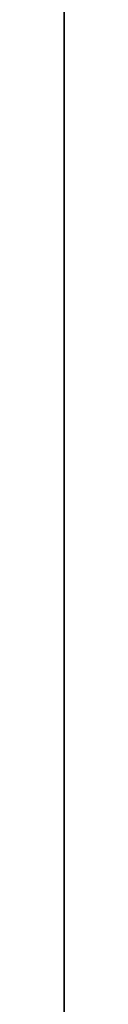
# Model space of a CAD drawing. Units: inches. Extents: x 2083 to 3317, y 1141 to 2115.
# Tile 74 of 256: x 2235.96 to 2235.96, y 1481.434 to 1485.751. Entities that reach past the tile are written whole.
import ezdxf

# ---------------------------------------------------------------- set-up
doc = ezdxf.new("R2010")
doc.units = ezdxf.units.IN
doc.layers.add('A-ANNO-DIMS', color=2, linetype='Continuous', lineweight=18)
doc.layers.add('A-WALL', color=7, linetype='Continuous', lineweight=35)
doc.layers.add('A-WALL-PATT', color=251, linetype='Continuous', lineweight=13, true_color=0x636466)
doc.styles.get("Standard").update_dxf_attribs({"font": 'arial.ttf'})
doc.dimstyles.new('ISO-25', dxfattribs={"dimtxt": 12, "dimasz": 12, "dimexe": 1.25, "dimexo": 0.625, "dimtad": 1, "dimlunit": 3, "dimtxsty": 'Standard', "dimcen": 2.5, "dimadec": 0, "dimazin": 0, "dimtfac": 1, "dimtmove": 0, "dimatfit": 3, "dimfxl": 1, "dimarcsym": 0})

# ---------------------------------------------------------------- blocks, each defined once
blk = doc.blocks.new('*D30')
at = {"layer": 'A-ANNO-DIMS', "color": 0, "lineweight": -2, "transparency": 16777216}
for p, q in [((2240.0179, 1445.2738), (2240.0179, 1448.0455)), ((2254.3293, 1445.2738), (2254.3293, 1448.0455)), ((2228.0179, 1446.7955), (2216.0179, 1446.7955)), ((2240.0179, 1446.7955), (2254.3293, 1446.7955)), ((2266.3293, 1446.7955), (2413.7649, 1446.7955))]:
    blk.add_line(p, q, dxfattribs=at)
at = {"layer": 'A-ANNO-DIMS', "color": 0, "transparency": 16777216}
for points in [[(2228.0179, 1448.7955), (2228.0179, 1444.7955), (2240.0179, 1446.7955)], [(2266.3293, 1448.7955), (2266.3293, 1444.7955), (2254.3293, 1446.7955)]]:
    blk.add_solid(points, dxfattribs=at)
at = {"layer": 'Defpoints', "color": 0, "transparency": 16777216}
for p in [(2254.3293, 1446.7955), (2240.0179, 1444.6488), (2254.3293, 1444.6488)]:
    blk.add_point(p, dxfattribs=at)
at = {"layer": 'A-ANNO-DIMS', "color": 0, "transparency": 16777216, "insert": (2346.0471, 1453.6252), "char_height": 12, "attachment_point": 5}
blk.add_mtext('WC 1\'-2 1/2" TYP.', dxfattribs=at)
blk = doc.blocks.new('*D31')
at = {"layer": 'A-ANNO-DIMS', "color": 0, "lineweight": -2, "transparency": 16777216}
for p, q in [((2237.8711, 1456.6488), (2237.8711, 1541.9152)), ((2239.3929, 1444.6488), (2236.6211, 1444.6488)), ((2237.8711, 1431.5475), (2237.8711, 1444.6488)), ((2239.3929, 1431.5475), (2236.6211, 1431.5475)), ((2237.8711, 1419.5475), (2237.8711, 1407.5475))]:
    blk.add_line(p, q, dxfattribs=at)
at = {"layer": 'A-ANNO-DIMS', "color": 0, "transparency": 16777216}
for points in [[(2235.8711, 1456.6488), (2239.8711, 1456.6488), (2237.8711, 1444.6488)], [(2235.8711, 1419.5475), (2239.8711, 1419.5475), (2237.8711, 1431.5475)]]:
    blk.add_solid(points, dxfattribs=at)
at = {"layer": 'Defpoints', "color": 0, "transparency": 16777216}
for p in [(2237.8711, 1444.6488), (2240.0179, 1444.6488), (2240.0179, 1431.5475)]:
    blk.add_point(p, dxfattribs=at)
at = {"layer": 'A-ANNO-DIMS', "color": 0, "transparency": 16777216, "insert": (2231.2175, 1505.282), "char_height": 12, "attachment_point": 5, "rotation": 90}
blk.add_mtext('1\'-1" TYP.', dxfattribs=at)
blk = doc.blocks.new('*D45')
at = {"layer": 'A-ANNO-DIMS', "color": 0, "lineweight": -2, "transparency": 16777216}
for p, q in [((2235.9598, 1478.3864), (2235.9598, 1531.3614)), ((2418.9598, 1478.3864), (2418.9598, 1531.3614)), ((2247.9598, 1530.1114), (2406.9598, 1530.1114))]:
    blk.add_line(p, q, dxfattribs=at)
at = {"layer": 'A-ANNO-DIMS', "color": 0, "transparency": 16777216}
for points in [[(2247.9598, 1532.1114), (2247.9598, 1528.1114), (2235.9598, 1530.1114)], [(2406.9598, 1532.1114), (2406.9598, 1528.1114), (2418.9598, 1530.1114)]]:
    blk.add_solid(points, dxfattribs=at)
at = {"layer": 'Defpoints', "color": 0, "transparency": 16777216}
for p in [(2418.9598, 1530.1114), (2235.9598, 1477.7614), (2418.9598, 1477.7614)]:
    blk.add_point(p, dxfattribs=at)
at = {"layer": 'A-ANNO-DIMS', "color": 0, "transparency": 16777216, "insert": (2327.4598, 1536.8673), "char_height": 12, "attachment_point": 5}
blk.add_mtext('15\'-3"', dxfattribs=at)
blk = doc.blocks.new('*D62')
at = {"layer": 'A-ANNO-DIMS', "color": 0, "lineweight": -2, "transparency": 16777216}
for p, q in [((2235.9598, 1469.3864), (2235.9598, 1522.3614)), ((2379.9598, 1469.3864), (2379.9598, 1522.3614)), ((2247.9598, 1521.1114), (2367.9598, 1521.1114))]:
    blk.add_line(p, q, dxfattribs=at)
at = {"layer": 'A-ANNO-DIMS', "color": 0, "transparency": 16777216}
for points in [[(2247.9598, 1523.1114), (2247.9598, 1519.1114), (2235.9598, 1521.1114)], [(2367.9598, 1523.1114), (2367.9598, 1519.1114), (2379.9598, 1521.1114)]]:
    blk.add_solid(points, dxfattribs=at)
at = {"layer": 'Defpoints', "color": 0, "transparency": 16777216}
for p in [(2379.9598, 1521.1114), (2235.9598, 1468.7614), (2379.9598, 1468.7614)]:
    blk.add_point(p, dxfattribs=at)
at = {"layer": 'A-ANNO-DIMS', "color": 0, "transparency": 16777216, "insert": (2307.9598, 1527.8632), "char_height": 12, "attachment_point": 5}
blk.add_mtext('12\'-0"', dxfattribs=at)

msp = doc.modelspace()

# ---------------------------------------------------------------- hatches: boundary and pattern name
at = {"layer": 'A-WALL-PATT'}
h = msp.add_hatch(color=256, dxfattribs=at)
h.dxf.hatch_style = 1
h.paths.add_polyline_path([(3126.9598, 2020.7614), (2748.9598, 2020.7614), (2604.9598, 2020.7614), (2226.9598, 2020.7614), (2226.9598, 1702.7614), (2466.9598, 1702.7614), (2466.9598, 1582.7614), (2418.9598, 1582.7614), (2418.9598, 1477.7614), (2226.9598, 1477.7614), (2226.9598, 1263.2614), (2544.9598, 1263.2614), (2544.9598, 1411.7614), (2604.9598, 1411.7614), (2685.9598, 1411.7614), (2685.9598, 1420.7614), (2604.9598, 1420.7614), (2604.9598, 1573.7614), (2604.9598, 1702.7614), (2604.9598, 2011.7614), (2748.9598, 2011.7614), (2748.9598, 1702.7614), (2862.9598, 1702.7614), (2862.9598, 1621.7614), (2871.9598, 1621.7614), (2871.9598, 1702.7614), (2883.9598, 1702.7614), (2883.9598, 1706.9395, -0.026459), (2883.9598, 1711.7614), (2757.9598, 1711.7614), (2757.9598, 1807.7614), (2787.9598, 1807.7614), (2787.9598, 1812.2614), (2757.9598, 1812.2614), (2757.9598, 2011.7614), (2877.9598, 2011.7614), (2877.9598, 1812.2614), (2847.9598, 1812.2614), (2847.9598, 1807.7614), (2889.8357, 1807.7614), (2889.8357, 1812.2614), (2882.4598, 1812.2614), (2882.4598, 2011.7614), (3117.9598, 2011.7614), (3117.9598, 1812.2614), (2937.8357, 1812.2614), (2937.8357, 1807.7614), (2995.7098, 1807.7614), (2995.7098, 1796.1177), (3000.2098, 1796.1177), (3000.2098, 1807.7614), (3117.9598, 1807.7614), (3117.9598, 1711.7614), (3000.2098, 1711.7614), (3000.2098, 1760.1177), (2998.5727, 1760.1177, -0.020711), (2995.7098, 1760.1177), (2995.7098, 1711.7614), (2931.9598, 1711.7614), (2931.9598, 1702.7614), (3126.9598, 1702.7614)])
h.paths.add_polyline_path([(2471.4598, 2011.7614), (2471.4598, 1810.0114), (2462.7169, 1810.0114), (2462.7169, 1805.5114), (2505.9598, 1805.5114), (2505.9598, 1810.0114), (2475.9598, 1810.0114), (2475.9598, 2011.7614), (2595.9598, 2011.7614), (2595.9598, 1810.0114), (2565.9598, 1810.0114), (2565.9598, 1805.5114), (2595.9598, 1805.5114), (2595.9598, 1711.7614), (2235.9598, 1711.7614), (2235.9598, 1805.5114), (2353.7098, 1805.5114), (2353.7098, 1796.0542), (2358.2098, 1796.0542), (2358.2098, 1805.5114), (2414.7169, 1805.5114), (2414.7169, 1810.0114), (2235.9598, 1810.0114), (2235.9598, 2011.7614)], flags=16)
h.paths.add_polyline_path([(2270.2047, 1994.61), (2270.2047, 1970.61), (2246.2047, 1970.61), (2246.2047, 1994.61)], flags=0)
edge = h.paths.add_edge_path(flags=0)
edge.add_ellipse((2332.0274, 1899.7982), major_axis=(-3.043, 3.043), ratio=0.168252, start_angle=-161.3322, end_angle=-156.3071, ccw=False)
edge.add_ellipse((2333.082, 1898.7435), major_axis=(-1.0546, 1.0546), ratio=0.453532, start_angle=-123.371, end_angle=-94.1591)
edge = h.paths.add_edge_path(flags=0)
edge.add_ellipse((2332.0274, 1968.8763), major_axis=(3.043, 3.043), ratio=0.168252, start_angle=18.6678, end_angle=23.6929)
edge.add_spline(control_points=[(2332.9256, 1970.6911), (2332.2268, 1970.3361), (2330.8937, 1969.6589), (2328.4131, 1970.9321), (2327.2039, 1967.7487), (2324.7096, 1969.9556), (2322.5328, 1967.0124), (2320.0128, 1971.2958), (2317.6803, 1968.1578), (2316.0405, 1967.102), (2315.4269, 1966.8096)], knot_values=[0, 0, 0, 0, 2.267059, 4.324559, 6.685584, 8.878641, 11.121502, 14.300359, 17.755284, 19.732645, 19.732645, 19.732645, 19.732645], degree=3, periodic=0)
edge.add_ellipse((2332.0274, 1968.8763), major_axis=(3.043, 3.043), ratio=0.168252, start_angle=18.6678, end_angle=23.6929, ccw=False)
edge.add_ellipse((2333.082, 1969.9309), major_axis=(1.0546, 1.0546), ratio=0.453532, start_angle=56.629, end_angle=85.8409, ccw=False)
edge = h.paths.add_edge_path(flags=0)
edge.add_spline(control_points=[(2296.4283, 1967.9879), (2293.6278, 1965.3363), (2287.7036, 1959.7271), (2299.7439, 1949.9957), (2294.5326, 1935.6685), (2290.5732, 1920.6035), (2293.3941, 1909.9737), (2296.1854, 1904.9665)], knot_values=[0.099185, 0.099185, 0.099185, 0.099185, 0.345301, 0.619822, 0.982653, 1.386093, 1.810555, 1.810555, 1.810555, 1.810555], degree=3, periodic=0)
edge.add_spline(control_points=[(2296.1854, 1904.9665), (2297.3836, 1902.6193), (2298.001, 1901.9493), (2298.553, 1901.4682)], knot_values=[0.006246, 0.006246, 0.006246, 0.006246, 0.055476, 0.055476, 0.055476, 0.055476], degree=3, periodic=0)
edge.add_spline(control_points=[(2298.553, 1901.4682), (2297.2586, 1900.9232), (2295.2253, 1900.2321), (2293.0602, 1900.6142), (2292.1014, 1900.7884), (2292.0896, 1900.7906)], knot_values=[0.312835, 0.312835, 0.312835, 0.312835, 0.40178, 0.474987, 0.475903, 0.475903, 0.475903, 0.475903], degree=3, periodic=0)
edge.add_arc((2292.7936, 1904.6641), 3.937, 215.4209, 259.6982, ccw=False)
edge.add_spline(control_points=[(2289.5853, 1902.3823), (2289.4767, 1902.5351), (2289.3685, 1902.688), (2289.2609, 1902.8412)], knot_values=[0.102872, 0.102872, 0.102872, 0.102872, 0.116896, 0.116896, 0.116896, 0.116896], degree=3, periodic=0)
edge.add_spline(control_points=[(2289.2609, 1902.8412), (2288.6866, 1902.5502), (2287.64, 1902.0199), (2285.8813, 1901.874), (2283.853, 1901.5044), (2281.72, 1899.7105), (2278.467, 1899.4929), (2276.1571, 1901.8832), (2272.259, 1899.8041), (2267.7776, 1901.8432), (2262.2439, 1900.184), (2257.4149, 1901.7821), (2254.3184, 1900.7261), (2253.1783, 1900.3373)], knot_values=[0, 0, 0, 0, 1.907977, 3.477176, 5.261074, 7.972851, 11.680248, 13.717921, 16.939592, 22.789562, 27.502503, 33.595215, 37.145618, 37.145618, 37.145618, 37.145618], degree=3, periodic=0)
edge.add_line((2253.1783, 1900.3373), (2250.2442, 1902.8412))
edge.add_line((2250.2442, 1902.8412), (2250.2442, 1965.8333))
edge.add_line((2250.2442, 1965.8333), (2253.1783, 1968.3371))
edge.add_spline(control_points=[(2253.1783, 1968.3371), (2254.3184, 1967.9483), (2257.4149, 1966.8924), (2262.2439, 1968.4904), (2267.7776, 1966.8313), (2271.5267, 1968.5372), (2273.8759, 1967.8283), (2274.2067, 1967.7276)], knot_values=[0, 0, 0, 0, 0.09018, 0.244935, 0.364644, 0.513233, 0.537855, 0.537855, 0.537855, 0.537855], degree=3, periodic=0)
edge.add_arc((2274.3529, 1963.7933), 3.937, 72.0511, 92.1279, ccw=False)
edge.add_arc((2281.2969, 1985.23), 18.5963, 252.05113, 288.56572)
edge.add_arc((2292.3167, 1956.0289), 12.6461, 71.02679, 113.77822, ccw=False)
edge = h.paths.add_edge_path(flags=0)
edge.add_spline(control_points=[(2274.8994, 1951.8562), (2275.0662, 1951.6166), (2275.2327, 1951.3766), (2275.398, 1951.1359)], knot_values=[1.409916, 1.409916, 1.409916, 1.409916, 1.43159, 1.43159, 1.43159, 1.43159], degree=3, periodic=0)
edge.add_spline(control_points=[(2275.398, 1951.1359), (2275.7921, 1950.5619), (2276.1792, 1949.9838), (2276.5455, 1949.3971)], knot_values=[1.358238, 1.358238, 1.358238, 1.358238, 1.409916, 1.409916, 1.409916, 1.409916], degree=3, periodic=0)
edge.add_line((2276.5455, 1949.3971), (2277.4373, 1947.8622))
edge.add_spline(control_points=[(2277.4373, 1947.8622), (2276.3038, 1945.6731), (2274.6397, 1942.4269), (2274.6316, 1938.0939), (2272.7991, 1930.8515), (2274.3564, 1943.897), (2275.9477, 1947.9234), (2276.5455, 1949.3971)], knot_values=[0.005632, 0.005632, 0.005632, 0.005632, 0.186014, 0.266002, 0.357087, 0.59639, 0.739732, 0.739732, 0.739732, 0.739732], degree=3, periodic=0)
edge.add_spline(control_points=[(2276.5455, 1949.3971), (2276.1792, 1949.9838), (2275.7921, 1950.5619), (2275.398, 1951.1359)], knot_values=[1.358238, 1.358238, 1.358238, 1.358238, 1.409916, 1.409916, 1.409916, 1.409916], degree=3, periodic=0)
edge.add_spline(control_points=[(2275.398, 1951.1359), (2274.9425, 1950.0805), (2274.2078, 1948.0253), (2273.9346, 1944.8515), (2272.4685, 1937.6275), (2273.4662, 1945.6965), (2274.7006, 1951.0595), (2274.8994, 1951.8562)], knot_values=[0.104364, 0.104364, 0.104364, 0.104364, 0.189636, 0.269624, 0.36071, 0.600013, 0.644622, 0.644622, 0.644622, 0.644622], degree=3, periodic=0)
h.paths.add_polyline_path([(2269.1675, 1963.1276, -0.357527), (2268.1706, 1960.9764, -0.092561), (2268.1706, 1939.4363, -0.357527), (2269.1675, 1937.2851, -0.357527), (2267.0163, 1938.282, -0.164785), (2254.6856, 1938.282, -0.357527), (2252.5344, 1937.2851, -0.357527), (2253.5313, 1939.4363, -0.092561), (2253.5313, 1960.9764, -0.357527), (2252.5344, 1963.1276, -0.357527), (2254.6856, 1962.1307, -0.164785), (2267.0163, 1962.1307, -0.357527)], flags=0)
h.paths.add_polyline_path([(2248.8741, 1967.8018), (2248.8741, 1957.0277), (2249.4578, 1957.0277), (2249.4578, 1911.6468), (2248.8741, 1911.6468), (2248.8741, 1900.8727), (2246.5119, 1900.8727, 0.197327), (2244.1497, 1902.4569), (2244.1497, 1966.2176, 0.197327), (2246.5119, 1967.8018)], flags=0)
h.paths.add_polyline_path([(2269.1675, 1931.3893, -0.357527), (2268.1706, 1929.2381, -0.092561), (2268.1706, 1907.6981, -0.357527), (2269.1675, 1905.5469, -0.357527), (2267.0163, 1906.5438, -0.164785), (2254.6856, 1906.5438, -0.357527), (2252.5344, 1905.5469, -0.357527), (2253.5313, 1907.6981, -0.092561), (2253.5313, 1929.2381, -0.357527), (2252.5344, 1931.3893, -0.357527), (2254.6856, 1930.3925, -0.164785), (2267.0163, 1930.3925, -0.357527)], flags=0)
edge = h.paths.add_edge_path(flags=0)
edge.add_spline(control_points=[(2276.1969, 1906.7237), (2276.1681, 1909.0289), (2276.114, 1913.3719), (2270.5984, 1924.925), (2273.9052, 1919.0128), (2275.9217, 1916.2621), (2275.4746, 1912.4021), (2277.2579, 1910.3806), (2276.696, 1908.225), (2276.6462, 1906.813), (2276.6178, 1906.0084)], knot_values=[0, 0, 0, 0, 8.61026, 16.221274, 18.843057, 23.804898, 27.440828, 29.356102, 31.203478, 33.650687, 33.650687, 33.650687, 33.650687], degree=3, periodic=0)
edge.add_spline(control_points=[(2276.6178, 1906.0084), (2276.6233, 1905.6241), (2276.4977, 1904.6287), (2275.4418, 1903.8547), (2274.9373, 1903.0804), (2274.8591, 1902.8412)], knot_values=[0.156488, 0.156488, 0.156488, 0.156488, 0.184398, 0.231376, 0.250598, 0.250598, 0.250598, 0.250598], degree=3, periodic=0)
edge.add_line((2274.8591, 1902.8412), (2276.506, 1902.8412))
edge.add_spline(control_points=[(2276.506, 1902.8412), (2276.7883, 1903.0849), (2277.6651, 1904.1252), (2278.2495, 1904.3407), (2277.6539, 1908.5274), (2278.1557, 1906.2278), (2278.1005, 1905.2859), (2278.8467, 1904.069), (2277.8568, 1903.4149), (2277.8742, 1902.991), (2277.9036, 1902.8412)], knot_values=[0.059574, 0.059574, 0.059574, 0.059574, 0.080753, 0.103741, 0.16972, 0.176036, 0.207137, 0.240474, 0.262341, 0.27366, 0.27366, 0.27366, 0.27366], degree=3, periodic=0)
edge.add_line((2277.9036, 1902.8412), (2280.0298, 1902.8412))
edge.add_spline(control_points=[(2280.0298, 1902.8412), (2279.8882, 1903.0884), (2279.4993, 1903.9816), (2280.1523, 1905.9393), (2278.1036, 1909.6578), (2279.7624, 1907.1853), (2280.3279, 1904.8749), (2280.4851, 1903.4896), (2281.4633, 1903.2494), (2281.7583, 1902.9365), (2281.834, 1902.8412)], knot_values=[0.013856, 0.013856, 0.013856, 0.013856, 0.034874, 0.088867, 0.107879, 0.126738, 0.158714, 0.193757, 0.217487, 0.226722, 0.226722, 0.226722, 0.226722], degree=3, periodic=0)
edge.add_spline(control_points=[(2281.834, 1902.8412), (2281.7875, 1902.8267), (2281.647, 1902.783), (2281.3955, 1902.8595), (2281.0881, 1902.9852), (2280.7207, 1903.0609), (2280.3335, 1903.0257), (2280.1248, 1902.8989), (2280.0298, 1902.8412)], knot_values=[0, 0, 0, 0, 0.14413, 0.435517, 0.749276, 1.153046, 1.548371, 1.878348, 1.878348, 1.878348, 1.878348], degree=3, periodic=0)
edge.add_line((2280.0298, 1902.8412), (2277.9036, 1902.8412))
edge.add_spline(control_points=[(2277.9036, 1902.8412), (2277.8929, 1902.7959), (2277.8654, 1902.6796), (2277.6075, 1902.6875), (2277.2741, 1902.8007), (2276.8379, 1902.6198), (2276.5838, 1902.7893), (2276.506, 1902.8412)], knot_values=[0, 0, 0, 0, 0.127189, 0.326199, 0.628009, 1.24357, 1.515331, 1.515331, 1.515331, 1.515331], degree=3, periodic=0)
edge.add_line((2276.506, 1902.8412), (2274.8591, 1902.8412))
edge.add_spline(control_points=[(2274.8591, 1902.8412), (2274.8144, 1902.8986), (2274.7251, 1903.0134), (2274.4935, 1903.119), (2274.2443, 1902.9605), (2273.9371, 1903.1849), (2273.614, 1902.9831), (2273.4083, 1902.883), (2273.3223, 1902.8412)], knot_values=[0, 0, 0, 0, 0.21843, 0.436957, 0.687977, 0.990379, 1.398396, 1.69185, 1.69185, 1.69185, 1.69185], degree=3, periodic=0)
edge.add_spline(control_points=[(2273.3223, 1902.8412), (2273.6167, 1903.4457), (2274.274, 1904.5383), (2276.0272, 1904.5737), (2276.207, 1906.5836), (2276.1969, 1906.7237)], knot_values=[0.012227, 0.012227, 0.012227, 0.012227, 0.059472, 0.106218, 0.134458, 0.134458, 0.134458, 0.134458], degree=3, periodic=0)
h.paths.add_polyline_path([(2270.7761, 1897.7898), (2270.7761, 1873.7898), (2246.7761, 1873.7898), (2246.7761, 1897.7898)], flags=0)
h.paths.add_polyline_path([(2353.7098, 1760.0051), (2353.7098, 1760.0542), (2358.2098, 1760.0542, -0.033729)], flags=0)
h.paths.add_polyline_path([(2321.8191, 1737.5292), (2341.9953, 1737.5292, -0.414214), (2343.2033, 1736.3212), (2343.2033, 1721.0206, -0.414214), (2341.9953, 1719.8127), (2321.8191, 1719.8127, -0.414214), (2320.6112, 1721.0206), (2320.6112, 1736.3212, -0.414214)], flags=0)
h.paths.add_polyline_path([(2324.235, 1736.3212), (2339.5794, 1736.3212, -0.414214), (2341.9953, 1733.9053), (2341.9953, 1725.4497, -0.414214), (2339.5794, 1723.0338), (2333.6806, 1723.0338), (2333.8453, 1722.0455, -0.870646), (2335.4254, 1721.8259, -0.767327), (2333.9227, 1721.4232), (2331.291, 1721.4232, -0.767327), (2329.7883, 1721.8259, -0.870646), (2331.3684, 1722.0455), (2331.5331, 1723.0338), (2324.235, 1723.0338, -0.414214), (2321.8191, 1725.4497), (2321.8191, 1733.9053, -0.414214)], flags=0)
h.paths.add_polyline_path([(2570.4838, 1928.6154), (2589.6838, 1928.6154), (2590.1688, 1928.6154), (2590.1688, 1904.9934), (2570.4838, 1904.9934)], flags=0)
h.paths.add_polyline_path([(2574.4473, 1927.2638, -1), (2572.8288, 1927.2638, -1)], flags=0)
h.paths.add_polyline_path([(2573.0899, 1926.9409), (2573.925, 1927.776), (2574.1477, 1927.5533), (2573.3126, 1926.7182)], flags=0)
h.paths.add_polyline_path([(2578.7791, 1919.7296, -1), (2571.5917, 1919.7296, -1)], flags=0)
h.paths.add_polyline_path([(2578.3854, 1919.7296, -1), (2571.9854, 1919.7296, -1)], flags=0)
h.paths.add_polyline_path([(2331.5958, 1729.4762, -1), (2333.618, 1729.4762, -1)], flags=0)
h.paths.add_polyline_path([(2578.0342, 1927.2638, -1), (2576.4157, 1927.2638, -1)], flags=0)
h.paths.add_polyline_path([(2576.6889, 1927.5311), (2576.9116, 1927.7538), (2577.7467, 1926.9186), (2577.524, 1926.6959)], flags=0)
h.paths.add_polyline_path([(2578.1391, 1909.8595, -1), (2572.2317, 1909.8595, -1)], flags=0)
h.paths.add_polyline_path([(2577.7454, 1909.8595, -1), (2572.6254, 1909.8595, -1)], flags=0)
h.paths.add_polyline_path([(2583.7977, 1927.2638, -1), (2582.1792, 1927.2638, -1)], flags=0)
h.paths.add_polyline_path([(2582.7186, 1927.7538), (2583.5538, 1926.9186), (2583.3311, 1926.6959), (2582.4959, 1927.5311)], flags=0)
h.paths.add_polyline_path([(2582.4959, 1927.5311), (2582.7186, 1927.7538), (2583.5538, 1926.9186), (2583.3311, 1926.6959)], flags=0)
h.paths.add_polyline_path([(2587.7391, 1920.5296, -1), (2581.8317, 1920.5296, -1)], flags=0)
h.paths.add_polyline_path([(2587.3454, 1920.5296, -1), (2582.2254, 1920.5296, -1)], flags=0)
h.paths.add_polyline_path([(2587.3846, 1927.2638, -1), (2585.7661, 1927.2638, -1)], flags=0)
h.paths.add_polyline_path([(2586.082, 1926.9802), (2586.9172, 1927.8154), (2587.1399, 1927.5927), (2586.3047, 1926.7575)], flags=0)
h.paths.add_polyline_path([(2588.3791, 1910.6595, -1), (2581.1917, 1910.6595, -1)], flags=0)
h.paths.add_polyline_path([(2587.9854, 1910.6595, -1), (2581.5854, 1910.6595, -1)], flags=0)
h.paths.add_polyline_path([(2417.1677, 1729.4779), (2437.3439, 1729.4779, -0.414214), (2438.5519, 1728.2699), (2438.5519, 1712.9693, -0.414214), (2437.3439, 1711.7614), (2417.1677, 1711.7614, -0.414214), (2415.9598, 1712.9693), (2415.9598, 1728.2699, -0.414214)], flags=0)
h.paths.add_polyline_path([(2419.5836, 1728.2699), (2434.928, 1728.2699, -0.414214), (2437.3439, 1725.8541), (2437.3439, 1717.3984, -0.414214), (2434.928, 1714.9825), (2429.0292, 1714.9825), (2429.1939, 1713.9942, -0.870646), (2430.774, 1713.7746, -0.767327), (2429.2713, 1713.372), (2426.6396, 1713.372, -0.767327), (2425.1369, 1713.7746, -0.870646), (2426.717, 1713.9942), (2426.8817, 1714.9825), (2419.5836, 1714.9825, -0.414214), (2417.1677, 1717.3984), (2417.1677, 1725.8541, -0.414214)], flags=0)
h.paths.add_polyline_path([(2419.5836, 1728.2699), (2434.928, 1728.2699, -0.414214), (2437.3439, 1725.8541), (2437.3439, 1717.3984, -0.414214), (2434.928, 1714.9825), (2429.0292, 1714.9825), (2428.3581, 1719.009), (2427.5528, 1719.009), (2426.8817, 1714.9825), (2419.5836, 1714.9825, -0.414214), (2417.1677, 1717.3984), (2417.1677, 1725.8541, -0.414214)], flags=0)
h.paths.add_polyline_path([(2426.9444, 1721.4249, -1), (2428.9666, 1721.4249, -1)], flags=0)
h.paths.add_polyline_path([(2475.9598, 1702.7614), (2595.9598, 1702.7614), (2595.9598, 1582.7614), (2475.9598, 1582.7614)], flags=16)
h.paths.add_polyline_path([(2427.9598, 1573.7614), (2595.9598, 1573.7614), (2595.9598, 1468.7614), (2595.9598, 1420.7614), (2384.4598, 1420.7614), (2384.4598, 1468.7614), (2427.9598, 1468.7614)], flags=16)
h.paths.add_polyline_path([(2379.9598, 1468.7614), (2379.9598, 1420.7614), (2235.9598, 1420.7614), (2235.9598, 1468.7614)], flags=16)
h.paths.add_polyline_path([(2317.816, 1466.6958), (2337.9922, 1466.6958, -0.414214), (2339.2002, 1465.4878), (2339.2002, 1450.1872, -0.414214), (2337.9922, 1448.9792), (2317.816, 1448.9792, -0.414214), (2316.6081, 1450.1872), (2316.6081, 1465.4878, -0.414214)], flags=0)
h.paths.add_polyline_path([(2320.2319, 1465.4878), (2335.5763, 1465.4878, -0.414214), (2337.9922, 1463.0719), (2337.9922, 1454.6163, -0.414214), (2335.5763, 1452.2004), (2329.6775, 1452.2004), (2329.8422, 1451.212, -0.870646), (2331.4223, 1450.9925, -0.767327), (2329.9196, 1450.5898), (2327.2879, 1450.5898, -0.767327), (2325.7852, 1450.9925, -0.870646), (2327.3653, 1451.212), (2327.53, 1452.2004), (2320.2319, 1452.2004, -0.414214), (2317.816, 1454.6163), (2317.816, 1463.0719, -0.414214)], flags=0)
h.paths.add_polyline_path([(2320.2319, 1465.4878), (2335.5763, 1465.4878, -0.414214), (2337.9922, 1463.0719), (2337.9922, 1454.6163, -0.414214), (2335.5763, 1452.2004), (2329.6775, 1452.2004), (2329.0064, 1456.2269), (2328.2011, 1456.2269), (2327.53, 1452.2004), (2320.2319, 1452.2004, -0.414214), (2317.816, 1454.6163), (2317.816, 1463.0719, -0.414214)], flags=0)
h.paths.add_polyline_path([(2327.5926, 1458.6428, -1), (2329.6148, 1458.6428, -1)], flags=0)
h.paths.add_polyline_path([(2244.4117, 1433.3405), (2241.9209, 1433.3405, -0.414214), (2240.0179, 1435.2435), (2240.0179, 1440.9528, -0.414211), (2241.9209, 1442.8559), (2244.4117, 1442.8559, -1.976472)], flags=0)
h.paths.add_polyline_path([(2245.3569, 1434.3975, -0.414214), (2245.3569, 1441.7988, -2.144098)], flags=0)
h.paths.add_polyline_path([(2535.9598, 1416.2614), (2535.9598, 1272.2614), (2235.9598, 1272.2614), (2235.9598, 1416.2614)], flags=16)
h.paths.add_polyline_path([(2260.1196, 1384.2928), (2260.1196, 1362.0386), (2237.8654, 1362.0386), (2237.8654, 1384.2928)], flags=0)
edge = h.paths.add_edge_path(flags=0)
edge.add_line((2318.2518, 1362.0933), (2318.1458, 1362.001))
edge.add_ellipse((2317.4451, 1360.431), major_axis=(2.8216, 2.8216), ratio=0.168252, start_angle=18.6678, end_angle=20.9481, ccw=False)
edge.add_ellipse((2318.423, 1361.409), major_axis=(0.9779, 0.9779), ratio=0.453532, start_angle=56.629, end_angle=70.2262, ccw=False)
edge = h.paths.add_edge_path(flags=0)
edge.add_line((2319.1074, 1295.5711), (2319.015, 1295.6771))
edge.add_ellipse((2317.4451, 1296.3778), major_axis=(-2.8216, 2.8216), ratio=0.168252, start_angle=-161.3322, end_angle=-159.0519, ccw=False)
edge.add_ellipse((2318.423, 1295.3999), major_axis=(-0.9779, 0.9779), ratio=0.453532, start_angle=-123.371, end_angle=-109.7738)
edge = h.paths.add_edge_path(flags=0)
edge.add_spline(control_points=[(2284.2103, 1301.1702), (2284.5807, 1300.4447), (2284.8912, 1299.892), (2285.1596, 1299.461)], knot_values=[0.039066, 0.039066, 0.039066, 0.039066, 0.055476, 0.055476, 0.055476, 0.055476], degree=3, periodic=0)
edge.add_line((2285.1596, 1299.461), (2284.2103, 1301.1702))
edge = h.paths.add_edge_path(flags=0)
edge.add_line((2280.4125, 1297.298), (2283.37, 1297.0361))
edge.add_line((2283.37, 1297.0361), (2286.4057, 1297.9263))
edge.add_spline(control_points=[(2286.4057, 1297.9263), (2285.3055, 1297.4631), (2284.3448, 1297.1292), (2283.37, 1297.0361)], knot_values=[0.394369, 0.394369, 0.394369, 0.394369, 0.475903, 0.475903, 0.475903, 0.475903], degree=3, periodic=0)
edge.add_spline(control_points=[(2283.37, 1297.0361), (2283.2814, 1297.0277), (2282.3163, 1296.9573), (2281.3125, 1297.1345), (2280.4234, 1297.296), (2280.4125, 1297.298)], knot_values=[0.312835, 0.312835, 0.312835, 0.312835, 0.320246, 0.393453, 0.394369, 0.394369, 0.394369, 0.394369], degree=3, periodic=0)
edge = h.paths.add_edge_path(flags=0)
edge.add_line((2284.4356, 1359.6073), (2280.4463, 1355.328))
edge.add_line((2280.4463, 1355.328), (2279.58, 1351.0178))
edge.add_line((2279.58, 1351.0178), (2282.413, 1346.5804))
edge.add_spline(control_points=[(2282.413, 1346.5804), (2283.1533, 1345.5892), (2284.2529, 1344.0289), (2284.801, 1342.3872), (2284.9352, 1341.8055)], knot_values=[1.240098, 1.240098, 1.240098, 1.240098, 1.332892, 1.382712, 1.382712, 1.382712, 1.382712], degree=3, periodic=0)
edge.add_spline(control_points=[(2284.9352, 1341.8055), (2285.3191, 1340.1406), (2285.233, 1338.4092), (2284.9099, 1336.6541)], knot_values=[1.097484, 1.097484, 1.097484, 1.097484, 1.240098, 1.240098, 1.240098, 1.240098], degree=3, periodic=0)
edge.add_spline(control_points=[(2284.9099, 1336.6541), (2284.5868, 1334.899), (2284.0267, 1333.1203), (2283.4626, 1331.3606)], knot_values=[0.95487, 0.95487, 0.95487, 0.95487, 1.097484, 1.097484, 1.097484, 1.097484], degree=3, periodic=0)
edge.add_line((2283.4626, 1331.3606), (2281.8904, 1326.1534))
edge.add_line((2281.8904, 1326.1534), (2280.7563, 1321.0561))
edge.add_line((2280.7563, 1321.0561), (2280.2992, 1316.002))
edge.add_line((2280.2992, 1316.002), (2280.7159, 1310.9501))
edge.add_line((2280.7159, 1310.9501), (2282.0281, 1305.9721))
edge.add_line((2282.0281, 1305.9721), (2284.2103, 1301.1702))
edge.add_spline(control_points=[(2284.2103, 1301.1702), (2283.3407, 1302.7302), (2282.6119, 1304.3365), (2282.0281, 1305.9721)], knot_values=[0.099185, 0.099185, 0.099185, 0.099185, 0.241799, 0.241799, 0.241799, 0.241799], degree=3, periodic=0)
edge.add_spline(control_points=[(2282.0281, 1305.9721), (2281.4443, 1307.6078), (2281.0055, 1309.2728), (2280.7159, 1310.9501)], knot_values=[0.241799, 0.241799, 0.241799, 0.241799, 0.384413, 0.384413, 0.384413, 0.384413], degree=3, periodic=0)
edge.add_spline(control_points=[(2280.7159, 1310.9501), (2280.4332, 1312.5876), (2280.2894, 1314.277), (2280.2989, 1315.962), (2280.2992, 1316.002)], knot_values=[0.384413, 0.384413, 0.384413, 0.384413, 0.523647, 0.527028, 0.527028, 0.527028, 0.527028], degree=3, periodic=0)
edge.add_spline(control_points=[(2280.2992, 1316.002), (2280.3123, 1317.687), (2280.4779, 1319.3679), (2280.7563, 1321.0561)], knot_values=[0.527028, 0.527028, 0.527028, 0.527028, 0.669642, 0.669642, 0.669642, 0.669642], degree=3, periodic=0)
edge.add_spline(control_points=[(2280.7563, 1321.0561), (2281.0346, 1322.7443), (2281.4259, 1324.4396), (2281.8904, 1326.1534)], knot_values=[0.669642, 0.669642, 0.669642, 0.669642, 0.812256, 0.812256, 0.812256, 0.812256], degree=3, periodic=0)
edge.add_spline(control_points=[(2281.8904, 1326.1534), (2282.2644, 1327.5333), (2282.7879, 1329.2618), (2283.3528, 1331.0178), (2283.4626, 1331.3606)], knot_values=[0.812256, 0.812256, 0.812256, 0.812256, 0.927087, 0.95487, 0.95487, 0.95487, 0.95487], degree=3, periodic=0)
edge.add_line((2283.4626, 1331.3606), (2284.9099, 1336.6541))
edge.add_line((2284.9099, 1336.6541), (2284.9352, 1341.8055))
edge.add_line((2284.9352, 1341.8055), (2282.413, 1346.5804))
edge.add_spline(control_points=[(2282.413, 1346.5804), (2281.2751, 1348.1038), (2280.0784, 1349.5703), (2279.58, 1351.0178)], knot_values=[1.382712, 1.382712, 1.382712, 1.382712, 1.525326, 1.525326, 1.525326, 1.525326], degree=3, periodic=0)
edge.add_spline(control_points=[(2279.58, 1351.0178), (2279.4433, 1351.4147), (2279.1363, 1352.8569), (2279.7352, 1354.2904), (2280.4463, 1355.328)], knot_values=[1.525326, 1.525326, 1.525326, 1.525326, 1.564439, 1.667941, 1.667941, 1.667941, 1.667941], degree=3, periodic=0)
edge.add_spline(control_points=[(2280.4463, 1355.328), (2281.4261, 1356.7578), (2282.9308, 1358.1826), (2284.4356, 1359.6073)], knot_values=[1.667941, 1.667941, 1.667941, 1.667941, 1.810555, 1.810555, 1.810555, 1.810555], degree=3, periodic=0)
edge.add_arc((2280.6231, 1348.5182), 11.7262, 71.02679, 113.77822)
edge.add_arc((2270.4049, 1375.5952), 17.2436, 252.05113, 288.56572, ccw=False)
edge.add_arc((2263.966, 1355.7178), 3.6506, 72.0511, 92.1279)
edge.add_arc((2263.966, 1355.7178), 3.6506, 92.1279, 177.9851)
edge.add_spline(control_points=[(2260.3176, 1355.8462), (2260.2604, 1354.2207), (2260.5513, 1350.1865), (2262.9993, 1346.7663), (2264.4727, 1344.649)], knot_values=[1.43159, 1.43159, 1.43159, 1.43159, 1.564144, 1.770695, 1.770695, 1.770695, 1.770695], degree=3, periodic=0)
edge.add_line((2264.4727, 1344.649), (2264.9356, 1343.9825))
edge.add_spline(control_points=[(2263.801, 1340.2481), (2263.8432, 1340.5141), (2264.0672, 1341.7565), (2264.5127, 1343.0025), (2264.935, 1343.9811)], knot_values=[0.53657, 0.53657, 0.53657, 0.53657, 0.559349, 0.644622, 0.644622, 0.644622, 0.644622], degree=3, periodic=0)
edge.add_spline(control_points=[(2264.935, 1343.9811), (2265.1178, 1343.715), (2265.2989, 1343.4479), (2265.4768, 1343.1794)], knot_values=[1.384077, 1.384077, 1.384077, 1.384077, 1.409916, 1.409916, 1.409916, 1.409916], degree=3, periodic=0)
edge.add_spline(control_points=[(2265.4768, 1343.1794), (2265.6546, 1342.9108), (2265.8293, 1342.6408), (2265.9991, 1342.3688)], knot_values=[1.358238, 1.358238, 1.358238, 1.358238, 1.384077, 1.384077, 1.384077, 1.384077], degree=3, periodic=0)
edge.add_line((2265.9991, 1342.3688), (2266.826, 1340.9455))
edge.add_spline(control_points=[(2266.826, 1340.9455), (2268.8944, 1337.0897), (2271.3982, 1325.843), (2270.5162, 1310.5686), (2275.9194, 1301.8606), (2277.7895, 1299.1994)], knot_values=[0.116896, 0.116896, 0.116896, 0.116896, 0.472987, 1.050969, 1.313793, 1.313793, 1.313793, 1.313793], degree=3, periodic=0)
edge.add_spline(control_points=[(2277.7895, 1299.1994), (2277.8394, 1299.1285), (2277.8894, 1299.0575), (2277.9396, 1298.9866)], knot_values=[0.109884, 0.109884, 0.109884, 0.109884, 0.116896, 0.116896, 0.116896, 0.116896], degree=3, periodic=0)
edge.add_line((2277.9396, 1298.9866), (2277.7888, 1299.1991))
edge.add_spline(control_points=[(2277.7888, 1299.1991), (2277.2566, 1298.9294), (2276.2864, 1298.4379), (2275.0394, 1298.3344), (2274.3833, 1298.2389), (2274.2153, 1298.2093)], knot_values=[33.12187, 33.12187, 33.12187, 33.12187, 35.029056, 36.598255, 37.144827, 37.144827, 37.144827, 37.144827], degree=3, periodic=0)
edge.add_line((2274.2153, 1298.2093), (2273.0731, 1297.893))
edge.add_spline(control_points=[(2273.0731, 1297.893), (2272.3229, 1297.5798), (2271.0392, 1296.5105), (2269.2484, 1296.2261), (2268.4231, 1296.3747)], knot_values=[26.532584, 26.532584, 26.532584, 26.532584, 29.198919, 31.839101, 31.839101, 31.839101, 31.839101], degree=3, periodic=0)
edge.add_line((2268.4231, 1296.3747), (2263.8785, 1297.4575))
edge.add_spline(control_points=[(2263.8785, 1297.4575), (2263.5561, 1297.3594), (2261.8603, 1296.8387), (2260.2388, 1297.2824), (2258.9335, 1297.5165)], knot_values=[15.919551, 15.919551, 15.919551, 15.919551, 16.939592, 21.226067, 21.226067, 21.226067, 21.226067], degree=3, periodic=0)
edge.add_line((2258.9335, 1297.5165), (2254.0552, 1297.329))
edge.add_spline(control_points=[(2254.0552, 1297.329), (2253.7555, 1297.2958), (2252.1137, 1297.1652), (2250.4619, 1297.5442), (2249.1297, 1297.6679)], knot_values=[5.306517, 5.306517, 5.306517, 5.306517, 6.276435, 10.613034, 10.613034, 10.613034, 10.613034], degree=3, periodic=0)
edge.add_line((2249.1297, 1297.6679), (2244.3316, 1296.8778))
edge.add_line((2244.3316, 1296.8778), (2241.611, 1299.1994))
edge.add_line((2241.611, 1299.1994), (2241.611, 1357.6094))
edge.add_line((2241.611, 1357.6094), (2244.3316, 1359.9311))
edge.add_line((2244.3316, 1359.9311), (2252.7288, 1359.5427))
edge.add_spline(control_points=[(2252.7288, 1359.5427), (2252.8709, 1359.5464), (2253.3057, 1359.5482), (2253.7398, 1359.5143), (2254.0317, 1359.4824)], knot_values=[0.233291, 0.233291, 0.233291, 0.233291, 0.244935, 0.268927, 0.268927, 0.268927, 0.268927], degree=3, periodic=0)
edge.add_line((2254.0317, 1359.4824), (2259.5872, 1359.4164))
edge.add_spline(control_points=[(2259.5872, 1359.4164), (2260.6771, 1359.6285), (2262.0732, 1359.897), (2263.5237, 1359.4593), (2263.8304, 1359.366)], knot_values=[0.422516, 0.422516, 0.422516, 0.422516, 0.513233, 0.537855, 0.537855, 0.537855, 0.537855], degree=3, periodic=0)
edge.add_arc((2263.966, 1355.7178), 3.6506, 72.0511, 92.1279, ccw=False)
edge.add_arc((2270.4049, 1375.5952), 17.2436, 252.05113, 288.56572)
edge.add_arc((2280.6231, 1348.5182), 11.7262, 71.02679, 113.77822, ccw=False)
h.paths.add_polyline_path([(2240.3405, 1359.4347), (2240.3405, 1349.4444), (2240.8818, 1349.4444), (2240.8818, 1307.3645), (2240.3405, 1307.3645), (2240.3405, 1297.3741), (2238.1502, 1297.3741, 0.197327), (2235.9598, 1298.8431), (2235.9598, 1357.9657, 0.197327), (2238.1502, 1359.4347)], flags=0)
h.paths.add_polyline_path([(2259.1578, 1355.1005, -0.357527), (2258.2334, 1353.1058, -0.092561), (2258.2334, 1333.1326, -0.357527), (2259.1578, 1331.1379, -0.357527), (2257.1631, 1332.0622, -0.164785), (2245.7293, 1332.0622, -0.357527), (2243.7346, 1331.1379, -0.357527), (2244.6589, 1333.1326, -0.092561), (2244.6589, 1353.1058, -0.357527), (2243.7346, 1355.1005, -0.357527), (2245.7293, 1354.1761, -0.164785), (2257.1631, 1354.1761, -0.357527)], flags=0)
edge = h.paths.add_edge_path(flags=0)
edge.add_line((2265.9991, 1342.3688), (2266.826, 1340.9455))
edge.add_line((2266.826, 1340.9455), (2265.3076, 1337.8141))
edge.add_line((2265.3076, 1337.8141), (2264.3582, 1334.6529))
edge.add_line((2264.3582, 1334.6529), (2264.262, 1333.7997))
edge.add_spline(control_points=[(2264.262, 1333.7997), (2264.2084, 1333.1871), (2264.1621, 1332.3655), (2264.0071, 1331.4139), (2263.969, 1331.2018)], knot_values=[0.464444, 0.464444, 0.464444, 0.464444, 0.516691, 0.531608, 0.531608, 0.531608, 0.531608], degree=3, periodic=0)
edge.add_spline(control_points=[(2263.969, 1331.2018), (2263.7745, 1330.1189), (2263.4244, 1328.7908), (2263.2574, 1328.5307), (2263.234, 1328.5146)], knot_values=[0.372682, 0.372682, 0.372682, 0.372682, 0.44885, 0.464444, 0.464444, 0.464444, 0.464444], degree=3, periodic=0)
edge.add_spline(control_points=[(2263.234, 1328.5146), (2263.0964, 1328.4202), (2263.1312, 1329.3015), (2263.275, 1330.6157)], knot_values=[0.280919, 0.280919, 0.280919, 0.280919, 0.372682, 0.372682, 0.372682, 0.372682], degree=3, periodic=0)
edge.add_spline(control_points=[(2263.275, 1330.6157), (2263.4187, 1331.93), (2263.6715, 1333.6773), (2263.9699, 1335.315)], knot_values=[0.189157, 0.189157, 0.189157, 0.189157, 0.280919, 0.280919, 0.280919, 0.280919], degree=3, periodic=0)
edge.add_spline(control_points=[(2263.9699, 1335.315), (2264.1005, 1336.0322), (2264.4188, 1337.6219), (2264.7548, 1338.8644), (2264.9474, 1339.4911)], knot_values=[0.097394, 0.097394, 0.097394, 0.097394, 0.137578, 0.189157, 0.189157, 0.189157, 0.189157], degree=3, periodic=0)
edge.add_spline(control_points=[(2264.9474, 1339.4911), (2265.29, 1340.6061), (2265.6442, 1341.494), (2265.9991, 1342.3688)], knot_values=[0.005632, 0.005632, 0.005632, 0.005632, 0.097394, 0.097394, 0.097394, 0.097394], degree=3, periodic=0)
h.paths.add_polyline_path([(2259.1578, 1325.671, -0.357527), (2258.2334, 1323.6763, -0.092561), (2258.2334, 1303.7031, -0.357527), (2259.1578, 1301.7084, -0.357527), (2257.1631, 1302.6327, -0.164785), (2245.7293, 1302.6327, -0.357527), (2243.7346, 1301.7084, -0.357527), (2244.6589, 1303.7031, -0.092561), (2244.6589, 1323.6763, -0.357527), (2243.7346, 1325.671, -0.357527), (2245.7293, 1324.7466, -0.164785), (2257.1631, 1324.7466, -0.357527)], flags=0)
edge = h.paths.add_edge_path(flags=0)
edge.add_spline(control_points=[(2261.7089, 1317.3114), (2261.6795, 1317.4176), (2261.7619, 1317.3885), (2262.4907, 1316.0899), (2262.9622, 1315.3009)], knot_values=[14.955861, 14.955861, 14.955861, 14.955861, 16.221274, 18.694826, 18.694826, 18.694826, 18.694826], degree=3, periodic=0)
edge.add_spline(control_points=[(2262.9622, 1315.3009), (2262.9904, 1315.2536), (2263.7021, 1314.0674), (2264.349, 1313.1272), (2264.7301, 1312.1642)], knot_values=[18.694826, 18.694826, 18.694826, 18.694826, 18.843057, 22.433791, 22.433791, 22.433791, 22.433791], degree=3, periodic=0)
edge.add_spline(control_points=[(2264.7301, 1312.1642), (2264.8756, 1311.7964), (2265.1769, 1310.7698), (2265.1431, 1309.5593), (2265.2477, 1308.8242)], knot_values=[22.433791, 22.433791, 22.433791, 22.433791, 23.804898, 26.172756, 26.172756, 26.172756, 26.172756], degree=3, periodic=0)
edge.add_line((2265.2477, 1308.8242), (2265.8508, 1307.1719))
edge.add_spline(control_points=[(2265.8508, 1307.1719), (2266.065, 1306.8217), (2266.3844, 1306.3322), (2266.4244, 1305.7805), (2266.4204, 1305.6112)], knot_values=[28.062562, 28.062562, 28.062562, 28.062562, 29.356102, 29.911721, 29.911721, 29.911721, 29.911721], degree=3, periodic=0)
edge.add_spline(control_points=[(2266.4204, 1305.6112), (2266.4161, 1305.4326), (2266.394, 1305.25), (2266.3648, 1305.0659)], knot_values=[29.911721, 29.911721, 29.911721, 29.911721, 30.497837, 30.497837, 30.497837, 30.497837], degree=3, periodic=0)
edge.add_line((2266.3648, 1305.0659), (2266.0662, 1302.1363))
edge.add_spline(control_points=[(2266.0662, 1302.1363), (2266.0712, 1301.78), (2265.9981, 1301.2), (2265.6633, 1300.759), (2265.5089, 1300.5859)], knot_values=[0.156488, 0.156488, 0.156488, 0.156488, 0.184398, 0.203543, 0.203543, 0.203543, 0.203543], degree=3, periodic=0)
edge.add_line((2265.5089, 1300.5859), (2264.4353, 1299.1994))
edge.add_line((2264.4353, 1299.1994), (2265.9624, 1299.1994))
edge.add_line((2265.9624, 1299.1994), (2267.336, 1301.1753))
edge.add_line((2267.336, 1301.1753), (2267.3117, 1301.9862))
edge.add_spline(control_points=[(2267.3117, 1301.9862), (2267.2611, 1302.8624), (2267.1602, 1303.7371), (2267.2715, 1303.3259)], knot_values=[0.126229, 0.126229, 0.126229, 0.126229, 0.166617, 0.166617, 0.166617, 0.166617], degree=3, periodic=0)
edge.add_spline(control_points=[(2267.2715, 1303.3259), (2267.28, 1303.2943), (2267.3098, 1303.1754), (2267.3735, 1302.8836), (2267.4061, 1302.6828), (2267.4179, 1302.601)], knot_values=[0.166617, 0.166617, 0.166617, 0.166617, 0.16972, 0.176036, 0.180765, 0.180765, 0.180765, 0.180765], degree=3, periodic=0)
edge.add_spline(control_points=[(2267.7439, 1300.9875), (2267.6876, 1301.1509), (2267.4805, 1301.6567), (2267.4838, 1302.1448), (2267.4179, 1302.601)], knot_values=[0.180765, 0.180765, 0.180765, 0.180765, 0.193767, 0.220139, 0.220139, 0.220139, 0.220139], degree=3, periodic=0)
edge.add_line((2267.4179, 1302.601), (2267.7439, 1300.9875))
edge.add_spline(control_points=[(2267.7439, 1300.9875), (2267.832, 1300.7319), (2267.932, 1300.3099), (2267.5548, 1299.9745), (2267.4294, 1299.8292)], knot_values=[0.220139, 0.220139, 0.220139, 0.220139, 0.240474, 0.25489, 0.25489, 0.25489, 0.25489], degree=3, periodic=0)
edge.add_line((2267.4294, 1299.8292), (2267.2584, 1299.1994))
edge.add_line((2267.2584, 1299.1994), (2269.23, 1299.1994))
edge.add_spline(control_points=[(2269.23, 1299.1994), (2269.0987, 1299.4287), (2268.8428, 1300.0163), (2269.0116, 1300.9159), (2268.9468, 1301.6607)], knot_values=[0.013856, 0.013856, 0.013856, 0.013856, 0.034874, 0.067073, 0.067073, 0.067073, 0.067073], degree=3, periodic=0)
edge.add_line((2268.9468, 1301.6607), (2268.4316, 1303.6031))
edge.add_spline(control_points=[(2268.4316, 1303.6031), (2268.1756, 1304.1924), (2267.5962, 1305.2513), (2268.0407, 1304.6232), (2268.2514, 1304.2824)], knot_values=[0.090155, 0.090155, 0.090155, 0.090155, 0.107879, 0.120289, 0.120289, 0.120289, 0.120289], degree=3, periodic=0)
edge.add_spline(control_points=[(2268.2514, 1304.2824), (2268.3609, 1304.1053), (2269.0578, 1302.918), (2269.3827, 1301.5904), (2269.5214, 1300.7759), (2269.5752, 1300.5558)], knot_values=[0.120289, 0.120289, 0.120289, 0.120289, 0.126738, 0.158714, 0.173506, 0.173506, 0.173506, 0.173506], degree=3, periodic=0)
edge.add_line((2269.5752, 1300.5558), (2270.6858, 1299.4213))
edge.add_spline(control_points=[(2270.6858, 1299.4213), (2270.7672, 1299.3573), (2270.8379, 1299.2814), (2270.9029, 1299.1994)], knot_values=[0.21816, 0.21816, 0.21816, 0.21816, 0.226722, 0.226722, 0.226722, 0.226722], degree=3, periodic=0)
edge.add_line((2270.9372, 1299.1929), (2270.9029, 1299.1994))
edge.add_spline(control_points=[(2270.9029, 1299.1994), (2270.8598, 1299.186), (2270.7295, 1299.1455), (2270.4963, 1299.2164), (2270.2717, 1299.3083), (2270.121, 1299.348), (2270.0633, 1299.3596)], knot_values=[0.939174, 0.939174, 0.939174, 0.939174, 1.083304, 1.374691, 1.68845, 1.878348, 1.878348, 1.878348, 1.878348], degree=3, periodic=0)
edge.add_line((2270.0633, 1299.3596), (2269.23, 1299.1994))
edge.add_line((2269.23, 1299.1994), (2267.2584, 1299.1994))
edge.add_spline(control_points=[(2267.2584, 1299.1994), (2267.2484, 1299.1574), (2267.223, 1299.0497), (2266.9838, 1299.0569), (2266.8092, 1299.1162), (2266.6769, 1299.1091), (2266.6365, 1299.1048)], knot_values=[0.757665, 0.757665, 0.757665, 0.757665, 0.884854, 1.083864, 1.385675, 1.515331, 1.515331, 1.515331, 1.515331], degree=3, periodic=0)
edge.add_spline(control_points=[(2266.6365, 1299.1048), (2266.4852, 1299.0888), (2266.2358, 1299.0171), (2266.0346, 1299.1513), (2265.9624, 1299.1994)], knot_values=[0, 0, 0, 0, 0.485905, 0.757665, 0.757665, 0.757665, 0.757665], degree=3, periodic=0)
edge.add_line((2265.9624, 1299.1994), (2264.4353, 1299.1994))
edge.add_line((2264.4353, 1299.1994), (2263.8584, 1299.3671))
edge.add_spline(control_points=[(2263.8584, 1299.3671), (2263.8189, 1299.3709), (2263.7795, 1299.3857), (2263.7401, 1299.4015)], knot_values=[0.845925, 0.845925, 0.845925, 0.845925, 0.978627, 0.978627, 0.978627, 0.978627], degree=3, periodic=0)
edge.add_line((2263.7218, 1299.3964), (2263.0103, 1299.1994))
edge.add_spline(control_points=[(2263.0103, 1299.1994), (2263.2458, 1299.6829), (2263.506, 1300.1281), (2263.8735, 1300.408)], knot_values=[0.012227, 0.012227, 0.012227, 0.012227, 0.052971, 0.052971, 0.052971, 0.052971], degree=3, periodic=0)
edge.add_spline(control_points=[(2263.8735, 1300.408), (2263.9321, 1300.4527), (2264.0842, 1300.553), (2264.2552, 1300.6242), (2264.3597, 1300.6647)], knot_values=[0.052971, 0.052971, 0.052971, 0.052971, 0.059472, 0.069086, 0.069086, 0.069086, 0.069086], degree=3, periodic=0)
edge.add_line((2264.3597, 1300.6647), (2265.1419, 1301.0778))
edge.add_line((2265.1419, 1301.0778), (2265.6758, 1302.7996))
edge.add_line((2265.6758, 1302.7996), (2265.5407, 1305.7041))
edge.add_line((2265.5407, 1305.7041), (2264.8031, 1309.3277))
edge.add_line((2264.8031, 1309.3277), (2263.0405, 1314.0918))
edge.add_spline(control_points=[(2263.0405, 1314.0918), (2262.3836, 1315.6714), (2261.796, 1316.9977), (2261.7089, 1317.3114)], knot_values=[11.216896, 11.216896, 11.216896, 11.216896, 14.955861, 14.955861, 14.955861, 14.955861], degree=3, periodic=0)
h.paths.add_polyline_path([(2871.9598, 1416.2614), (2895.91, 1416.2614), (2895.91, 1420.7614), (2871.9598, 1420.7614), (2871.9598, 1501.7614), (2862.9598, 1501.7614), (2862.9598, 1420.7614), (2805.9598, 1420.7614), (2805.9598, 1411.7614), (2862.9598, 1411.7614), (2862.9598, 1263.2614), (3126.9598, 1263.2614), (3126.9598, 1411.7614), (3126.9598, 1486.7614), (2943.9598, 1486.7614), (2943.9598, 1477.7614), (2967.8603, 1477.7614), (2967.8603, 1420.7614), (2943.91, 1420.7614), (2943.91, 1416.2614), (3117.9598, 1416.2614), (3117.9598, 1420.7614), (2972.3603, 1420.7614), (2972.3603, 1477.7614), (3117.9598, 1477.7614), (3117.9598, 1420.7614), (3117.9598, 1272.2614), (2871.9598, 1272.2614)], flags=0)
h.paths.add_polyline_path([(2457.1256, 1485.9425), (2527.6027, 1485.9425), (2527.6027, 1537.6357), (2457.1256, 1537.6357)], flags=8)
h.paths.add_polyline_path([(2481.0051, 1609.9818), (2590.7658, 1609.9818), (2590.7658, 1682.0034), (2481.0051, 1682.0034)], flags=8)
h.paths.add_polyline_path([(2483.085, 1729.1268), (2553.562, 1729.1268), (2553.562, 1780.82), (2483.085, 1780.82)], flags=8)

# ---------------------------------------------------------------- linework, layer by layer
at = {"layer": 'A-WALL'}
msp.add_line((2235.9598, 1702.7614), (2235.9598, 1477.7614), dxfattribs=at)
msp.add_line((2235.9598, 1702.7614), (2235.9598, 1477.7614), dxfattribs=at)

# ---------------------------------------------------------------- dimensions: what is measured, and where the dimension line sits
at = {"layer": 'A-ANNO-DIMS'}
for base, p1, p2, picture, middle in [((2418.9598, 1530.1114), (2235.9598, 1477.7614), (2418.9598, 1477.7614), '*D45', (2327.4598, 1536.8673)), ((2379.9598, 1521.1114), (2235.9598, 1468.7614), (2379.9598, 1468.7614), '*D62', (2307.9598, 1527.8632))]:
    dim = msp.add_linear_dim(base=base, p1=p1, p2=p2, dimstyle='ISO-25', override={"dimdec": 1, "dimlfac": 1, "dimrnd": 0, "dimzin": 1, "dimdsep": 46, "dimlunit": 4, "dimfrac": 2}, dxfattribs=at)
    dim.commit()
    dim.dimension.update_dxf_attribs({"geometry": picture, "text_midpoint": middle})
dim = msp.add_linear_dim(base=(2237.8711, 1444.6488), p1=(2240.0179, 1431.5475), p2=(2240.0179, 1444.6488), angle=90, text='<> TYP.', dimstyle='ISO-25', override={"dimdec": 1, "dimlfac": 1, "dimrnd": 0, "dimzin": 1, "dimdsep": 46, "dimlunit": 4, "dimfrac": 2}, dxfattribs=at)
dim.commit()
dim.dimension.update_dxf_attribs({"geometry": '*D31', "text_midpoint": (2231.2175, 1505.282)})
dim = msp.add_linear_dim(base=(2254.3293, 1446.7955), p1=(2240.0179, 1444.6488), p2=(2254.3293, 1444.6488), text='WC <> TYP.', dimstyle='ISO-25', override={"dimdec": 1, "dimlfac": 1, "dimrnd": 0, "dimzin": 1, "dimdsep": 46, "dimlunit": 4, "dimfrac": 2}, dxfattribs=at)
dim.commit()
dim.dimension.update_dxf_attribs({"geometry": '*D30', "text_midpoint": (2346.0471, 1453.6252)})

doc.saveas('drawing.dxf')
